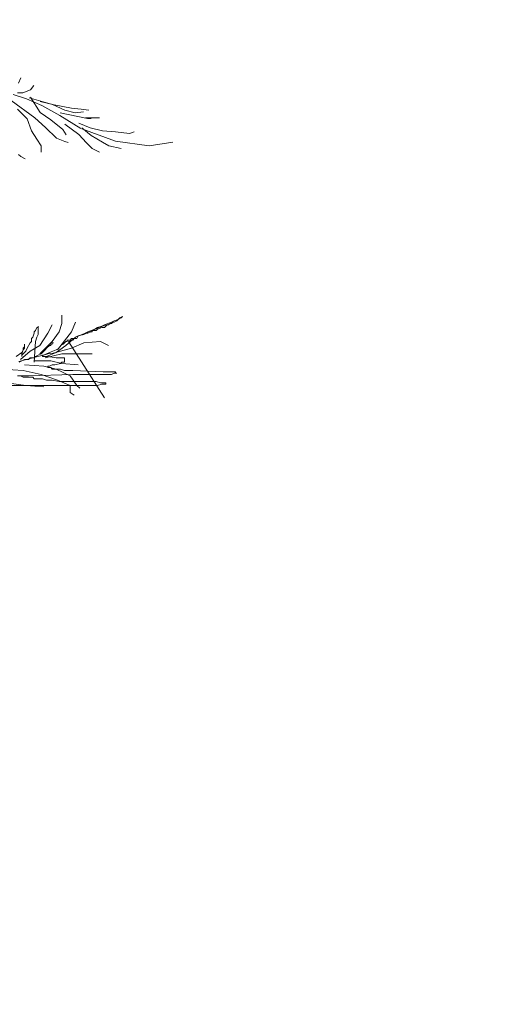
# Model space of a CAD drawing. Units: millimetres. Extents: x 595116 to 630915, y 909473 to 920225.
# Tile 63 of 134: x 629608.93 to 629618.94, y 919281.16 to 919301.58. Entities that reach past the tile are written whole.
import ezdxf

# ---------------------------------------------------------------- set-up
doc = ezdxf.new("R2010")
doc.units = ezdxf.units.MM
doc.layers.add('Dimension', color=3, linetype='Continuous', lineweight=18)
doc.layers.add('L-PLNT', color=85, linetype='Continuous', lineweight=13)
doc.styles.get("Standard").update_dxf_attribs({"font": 'arial.ttf'})
doc.dimstyles.new('ISO-25', dxfattribs={"dimtxt": 9, "dimasz": 6, "dimexe": 1.25, "dimexo": 0.625, "dimtad": 1, "dimlunit": 4, "dimtxsty": 'Standard', "dimcen": 2.5, "dimadec": 0, "dimazin": 0, "dimtfac": 1, "dimtmove": 0, "dimatfit": 3, "dimfxl": 1, "dimarcsym": 0})

# ---------------------------------------------------------------- blocks, each defined once
blk = doc.blocks.new('A$C4FB75ABC')
for p, q in [((4.5963, 3.4774), (4.6082, 3.5072)), ((4.6201, 3.4238), (4.6619, 3.4416)), ((4.6619, 3.4416), (4.6798, 3.4655)), ((4.5545, 3.382), (4.6858, 3.2866)), ((4.5657, 3.4153), (4.6395, 3.3917)), ((4.5903, 3.4238), (4.6201, 3.4238)), ((4.6395, 3.3917), (4.7247, 3.3534)), ((4.6551, 3.396), (4.7847, 3.3597)), ((4.6619, 3.3999), (4.7156, 3.3164)), ((4.7156, 3.3761), (4.7931, 3.3582)), ((4.5903, 3.3343), (4.644, 3.2807)), ((4.7247, 3.3534), (4.8242, 3.2989)), ((4.7847, 3.3597), (4.8521, 3.3286)), ((4.7931, 3.3582), (4.8886, 3.3403)), ((4.8521, 3.3286), (4.9091, 3.3131)), ((4.8886, 3.3403), (4.9422, 3.3343)), ((4.9422, 3.3343), (4.984, 3.3284)), ((4.644, 3.2807), (4.6679, 3.2151)), ((4.6858, 3.2866), (4.7454, 3.233)), ((4.7156, 3.3164), (4.7752, 3.2747)), ((4.7752, 3.2747), (4.8408, 3.2211)), ((4.8242, 3.2989), (4.9411, 3.2265)), ((4.8262, 3.3131), (4.9765, 3.282)), ((4.9091, 3.3131), (4.9558, 3.3183)), ((4.9661, 3.2866), (5.0079, 3.2866)), ((4.9765, 3.282), (4.9973, 3.282)), ((5.0079, 3.2866), (5.0437, 3.2866)), ((4.6679, 3.2151), (4.6977, 3.1674)), ((4.7454, 3.233), (4.8051, 3.1734)), ((4.8408, 3.2211), (4.8587, 3.1912)), ((4.8521, 3.2509), (4.9299, 3.1939)), ((4.9299, 3.2561), (4.9921, 3.2302)), ((4.9454, 3.2302), (4.9973, 3.1887)), ((4.9454, 3.225), (5.1321, 3.1576)), ((4.9921, 3.2302), (5.0595, 3.2146)), ((5.0595, 3.2146), (5.1321, 3.2094)), ((4.6977, 3.1674), (4.7215, 3.1316)), ((4.8051, 3.1734), (4.8528, 3.1555)), ((4.9299, 3.1939), (4.9713, 3.1472)), ((4.9973, 3.1887), (5.0595, 3.1524)), ((5.1321, 3.2094), (5.2099, 3.1991)), ((5.1321, 3.1576), (5.3187, 3.1317)), ((5.2099, 3.1991), (5.2358, 3.2094)), ((4.7215, 3.1316), (4.7215, 3.0959)), ((4.8528, 3.1555), (4.8707, 3.1495)), ((4.9713, 3.1472), (5.0025, 3.1162)), ((5.0025, 3.1162), (5.0439, 3.0954)), ((5.0595, 3.1524), (5.0958, 3.1317)), ((5.0958, 3.1317), (5.1632, 3.1162)), ((5.3187, 3.1317), (5.4484, 3.1524)), ((4.5963, 3.0839), (4.6082, 3.072)), ((4.6082, 3.072), (4.6321, 3.0601)), ((4.835, 2.1495), (4.835, 2.1952)), ((5.1477, 2.1724), (5.1629, 2.18)), ((5.1553, 2.18), (5.1477, 2.1724)), ((5.1706, 2.1876), (5.1553, 2.18)), ((5.1629, 2.18), (5.1706, 2.1876)), ((4.6901, 2.1114), (4.6977, 2.1266)), ((4.6977, 2.1266), (4.7054, 2.1266)), ((4.7054, 2.1266), (4.7054, 2.1343)), ((4.7054, 2.1343), (4.7054, 2.0885)), ((4.7587, 2.0961), (4.7816, 2.1419)), ((4.8198, 2.1038), (4.835, 2.1495)), ((4.8884, 2.1038), (4.9113, 2.1571)), ((4.9113, 2.0733), (5.079, 2.1419)), ((5.0333, 2.1266), (5.018, 2.119)), ((5.0562, 2.1343), (5.0333, 2.1266)), ((5.0333, 2.119), (5.0562, 2.1266)), ((5.0714, 2.1419), (5.0562, 2.1343)), ((5.0562, 2.1266), (5.0714, 2.1266)), ((5.1095, 2.1571), (5.0714, 2.1419)), ((5.0714, 2.1266), (5.079, 2.1343)), ((5.079, 2.1343), (5.0867, 2.1419)), ((5.0867, 2.1419), (5.0943, 2.1419)), ((5.0943, 2.1419), (5.1019, 2.1495)), ((5.1019, 2.1495), (5.1095, 2.1495)), ((5.1248, 2.1648), (5.1095, 2.1571)), ((5.1095, 2.1495), (5.1172, 2.1571)), ((5.1172, 2.1571), (5.1248, 2.1571)), ((5.1477, 2.1724), (5.1248, 2.1648)), ((5.1248, 2.1571), (5.1401, 2.1648)), ((5.1401, 2.1648), (5.1477, 2.1724)), ((4.6672, 2.0657), (4.6749, 2.0733)), ((4.6749, 2.0733), (4.6825, 2.0961)), ((4.6825, 2.1038), (4.6901, 2.1114)), ((4.6825, 2.0961), (4.6825, 2.1038)), ((4.6977, 2.0733), (4.6901, 2.0504)), ((4.7054, 2.0885), (4.6977, 2.0733)), ((4.713, 2.0275), (4.7587, 2.0961)), ((4.7816, 2.0504), (4.8198, 2.1038)), ((4.8121, 2.0047), (4.8884, 2.1038)), ((4.8579, 2.0275), (4.9113, 2.0733)), ((4.9036, 2.0657), (4.9113, 2.0733)), ((4.9113, 2.0733), (4.9265, 2.0809)), ((4.9265, 2.0809), (4.9189, 2.0657)), ((4.9265, 2.0809), (4.957, 2.0885)), ((4.9494, 2.0885), (4.9265, 2.0809)), ((4.9799, 2.1038), (4.9494, 2.0885)), ((4.957, 2.0885), (4.9723, 2.0961)), ((4.9723, 2.0961), (4.9799, 2.0961)), ((5.018, 2.119), (4.9799, 2.1038)), ((4.9799, 2.0961), (4.9952, 2.1038)), ((4.9952, 2.1038), (5.0028, 2.1038)), ((5.0028, 2.1038), (5.0028, 2.1114)), ((5.0028, 2.1114), (5.0257, 2.1114)), ((5.0257, 2.1114), (5.0333, 2.119)), ((4.6215, 2.0123), (4.6291, 2.0199)), ((4.6291, 2.0199), (4.6291, 2.0352)), ((4.6291, 2.0352), (4.6291, 2.0123)), ((4.6444, 2.0123), (4.6596, 2.0428)), ((4.6596, 2.0428), (4.6672, 2.0504)), ((4.6596, 1.9971), (4.713, 2.0275)), ((4.6672, 2.0504), (4.6672, 2.0657)), ((4.6901, 2.0504), (4.6825, 1.9361)), ((4.713, 1.9818), (4.7816, 2.0504)), ((4.7664, 2.0275), (4.7511, 2.0123)), ((4.774, 2.0275), (4.7664, 2.0275)), ((4.7816, 2.0352), (4.774, 2.0352)), ((4.774, 2.0352), (4.774, 2.0275)), ((4.7892, 2.0428), (4.7816, 2.0428)), ((4.7816, 2.0428), (4.7816, 2.0352)), ((4.8045, 1.9894), (4.8579, 2.0275)), ((4.8198, 2.0123), (4.8274, 2.0275)), ((4.8274, 2.0275), (4.8426, 2.0352)), ((4.8426, 2.0352), (4.8579, 2.0504)), ((4.8579, 2.0504), (4.8655, 2.0504)), ((4.8655, 2.0504), (4.8655, 2.058)), ((4.8655, 2.058), (4.8808, 2.058)), ((4.8808, 2.0504), (4.8731, 2.0504)), ((4.8731, 2.0504), (5.0714, 1.7379)), ((4.8808, 2.058), (4.8884, 2.0657)), ((4.896, 2.058), (4.8808, 2.058)), ((4.8808, 2.058), (4.8808, 2.0504)), ((4.8884, 2.0657), (4.9036, 2.0657)), ((4.8884, 2.0123), (4.957, 2.0428)), ((4.9036, 2.0657), (4.896, 2.058)), ((4.9189, 2.0657), (4.9036, 2.0657)), ((4.957, 2.0428), (5.0485, 2.0504)), ((5.0485, 2.0504), (5.0943, 2.0275)), ((4.5833, 1.9666), (4.6138, 1.9894)), ((4.7725, 1.9851), (4.5975, 1.9398)), ((4.6062, 1.9513), (4.6596, 1.9971)), ((4.6138, 1.9894), (4.6215, 2.0047)), ((4.6215, 2.0047), (4.6138, 1.9818)), ((4.6138, 1.9818), (4.6138, 1.9666)), ((4.6138, 1.9742), (4.6215, 1.9818)), ((4.6138, 1.9666), (4.6138, 1.9742)), ((4.6215, 2.0047), (4.6215, 2.0123)), ((4.6291, 2.0123), (4.6215, 2.0047)), ((4.6215, 1.9818), (4.6367, 1.9971)), ((4.6367, 1.9971), (4.6444, 2.0123)), ((4.6596, 1.9589), (4.652, 1.9513)), ((4.6825, 1.9589), (4.6596, 1.9589)), ((4.6901, 1.9666), (4.6825, 1.9589)), ((4.7054, 1.9742), (4.6901, 1.9666)), ((4.7206, 1.9818), (4.7054, 1.9742)), ((4.7359, 1.9971), (4.7206, 1.9818)), ((4.7282, 1.9666), (4.7282, 1.9742)), ((4.7282, 1.9742), (4.7359, 1.9742)), ((4.7587, 1.9666), (4.7282, 1.9666)), ((4.7435, 2.0047), (4.7359, 1.9971)), ((4.7359, 1.9742), (4.7511, 1.9818)), ((4.7511, 2.0123), (4.7435, 2.0047)), ((4.7435, 1.9589), (4.835, 1.9818)), ((4.7511, 1.9818), (4.7664, 1.9894)), ((4.7511, 1.9666), (4.8045, 1.9894)), ((4.8045, 1.9589), (4.7587, 1.9666)), ((4.7664, 1.9894), (4.8045, 2.0047)), ((4.774, 1.9818), (4.8884, 2.0123)), ((4.8045, 2.0047), (4.8198, 2.0123)), ((4.8503, 1.9589), (4.8045, 1.9589)), ((4.835, 1.9818), (4.9494, 1.9818)), ((4.8503, 1.9361), (4.8503, 1.9589)), ((4.9494, 1.9818), (5.0028, 1.9818)), ((4.6138, 1.9437), (4.5986, 1.9361)), ((4.6291, 1.9513), (4.6138, 1.9437)), ((4.652, 1.9513), (4.6291, 1.9513)), ((4.6291, 1.9208), (4.7359, 1.9132)), ((4.6825, 1.9437), (4.774, 1.9437)), ((4.7359, 1.9132), (4.8045, 1.898)), ((4.7587, 1.9056), (4.7587, 1.9132)), ((4.7587, 1.9132), (4.7664, 1.9132)), ((4.774, 1.9056), (4.7587, 1.9056)), ((4.7664, 1.9132), (4.7816, 1.9208)), ((4.774, 1.9437), (4.835, 1.9285)), ((4.7816, 1.898), (4.774, 1.9056)), ((4.7816, 1.9208), (4.7969, 1.9208)), ((4.7969, 1.9208), (4.8274, 1.9285)), ((4.8274, 1.9285), (4.835, 1.9361)), ((4.835, 1.9361), (4.8503, 1.9361)), ((4.835, 1.9285), (4.9265, 1.9208)), ((4.5071, 1.898), (4.6215, 1.8903)), ((4.6062, 1.8599), (4.591, 1.8599)), ((4.591, 1.8599), (4.652, 1.8599)), ((4.6215, 1.8522), (4.6062, 1.8599)), ((4.6215, 1.8903), (4.7206, 1.8675)), ((4.6749, 1.8522), (4.6215, 1.8522)), ((4.652, 1.8599), (4.896, 1.8675)), ((4.6825, 1.8446), (4.6749, 1.8522)), ((4.7206, 1.8675), (4.8121, 1.837)), ((4.8274, 1.898), (4.7816, 1.898)), ((4.8045, 1.898), (4.8808, 1.8599)), ((4.8503, 1.8903), (4.8274, 1.898)), ((4.896, 1.8903), (4.8503, 1.8903)), ((4.8808, 1.8599), (4.9189, 1.8065)), ((5.0638, 1.8827), (4.896, 1.8903)), ((4.896, 1.8675), (5.1095, 1.8675)), ((5.1324, 1.8827), (5.0638, 1.8827)), ((5.1095, 1.8675), (5.1248, 1.8751)), ((5.1248, 1.8751), (5.1401, 1.8751)), ((5.1324, 1.8751), (5.1324, 1.8827)), ((5.1401, 1.8751), (5.1324, 1.8751)), ((4.1639, 1.8065), (5.0333, 1.8065)), ((4.53, 1.8217), (4.6367, 1.8065)), ((4.6367, 1.8065), (4.7359, 1.7989)), ((4.7282, 1.8446), (4.6825, 1.8446)), ((4.7511, 1.837), (4.7282, 1.8446)), ((4.7816, 1.837), (4.7511, 1.837)), ((4.8198, 1.8294), (4.7816, 1.837)), ((4.8121, 1.837), (4.8808, 1.8065)), ((5.0257, 1.8294), (4.8198, 1.8294)), ((4.8808, 1.8065), (4.8808, 1.7684)), ((4.9189, 1.8065), (4.9341, 1.7913)), ((5.0485, 1.8217), (5.0257, 1.8294)), ((5.0333, 1.8065), (5.0562, 1.8141)), ((5.079, 1.8217), (5.0485, 1.8217)), ((5.0562, 1.8141), (5.079, 1.8141)), ((5.079, 1.8141), (5.079, 1.8217)), ((4.8808, 1.7684), (4.9036, 1.7531))]:
    blk.add_line(p, q)
blk = doc.blocks.new('*D210')
at = {"layer": 'Defpoints', "color": 0, "transparency": 16777216}
for p in [(629586.227, 919310.123), (629593.946, 919310.123), (629586.227, 919258.662)]:
    blk.add_point(p, dxfattribs=at)
at = {"layer": 'Dimension', "color": 0, "lineweight": -2, "transparency": 16777216}
for p, q in [((629593.946, 919310.123), (629593.946, 919449.69)), ((629586.852, 919310.123), (629595.196, 919310.123)), ((629593.946, 919264.662), (629593.946, 919304.123)), ((629586.852, 919258.662), (629595.196, 919258.662))]:
    blk.add_line(p, q, dxfattribs=at)
at = {"layer": 'Dimension', "color": 0, "transparency": 16777216}
for points in [[(629592.946, 919304.123), (629594.946, 919304.123), (629593.946, 919310.123)], [(629592.946, 919264.662), (629594.946, 919264.662), (629593.946, 919258.662)]]:
    blk.add_solid(points, dxfattribs=at)
at = {"layer": 'Dimension', "color": 0, "transparency": 16777216, "insert": (629588.662, 919382.907), "char_height": 9, "attachment_point": 5, "rotation": 90}
blk.add_mtext('CANOPY 4\'-3 1/2" TYP.', dxfattribs=at)
blk = doc.blocks.new('*D216')
at = {"layer": 'Defpoints', "color": 0, "transparency": 16777216}
for p in [(629743.541, 919411.928), (629505.041, 919411.828), (629743.541, 918832.378)]:
    blk.add_point(p, dxfattribs=at)
at = {"layer": 'Dimension', "color": 0, "lineweight": -2, "transparency": 16777216}
for p, q in [((629743.541, 919411.303), (629743.541, 918831.128)), ((629505.041, 919411.203), (629505.041, 918831.128)), ((629511.041, 918832.378), (629737.541, 918832.378))]:
    blk.add_line(p, q, dxfattribs=at)
at = {"layer": 'Dimension', "color": 0, "transparency": 16777216}
for points in [[(629511.041, 918833.378), (629511.041, 918831.378), (629505.041, 918832.378)], [(629737.541, 918833.378), (629737.541, 918831.378), (629743.541, 918832.378)]]:
    blk.add_solid(points, dxfattribs=at)
at = {"layer": 'Dimension', "color": 0, "transparency": 16777216, "insert": (629624.291, 918837.656), "char_height": 9, "attachment_point": 5}
blk.add_mtext('19\'-10 1/2"', dxfattribs=at)

msp = doc.modelspace()

# ---------------------------------------------------------------- block references
at = {"layer": 'L-PLNT', "xscale": 3.753413438031968, "yscale": 3.753413438031968, "zscale": 3.753413438031968}
msp.add_blockref('A$C4FB75ABC', (629591.653, 919287.212), dxfattribs=at)

# ---------------------------------------------------------------- dimensions: what is measured, and where the dimension line sits
at = {"layer": 'Dimension'}
dim = msp.add_linear_dim(base=(629593.946, 919310.123), p1=(629586.227, 919258.662), p2=(629586.227, 919310.123), angle=90, text='CANOPY <> TYP.', dimstyle='ISO-25', override={"dimdec": 1, "dimlfac": 1, "dimrnd": 0, "dimzin": 1, "dimdsep": 46, "dimlunit": 4, "dimfrac": 2}, dxfattribs=at)
dim.commit()
dim.dimension.update_dxf_attribs({"geometry": '*D210', "text_midpoint": (629588.662, 919382.907)})
dim = msp.add_linear_dim(base=(629743.541, 918832.378), p1=(629505.041, 919411.828), p2=(629743.541, 919411.928), dimstyle='ISO-25', override={"dimdec": 1, "dimlfac": 1, "dimrnd": 0, "dimzin": 1, "dimdsep": 46, "dimlunit": 4, "dimfrac": 2}, dxfattribs=at)
dim.commit()
dim.dimension.update_dxf_attribs({"geometry": '*D216', "text_midpoint": (629624.291, 918837.656)})

doc.saveas('drawing.dxf')
